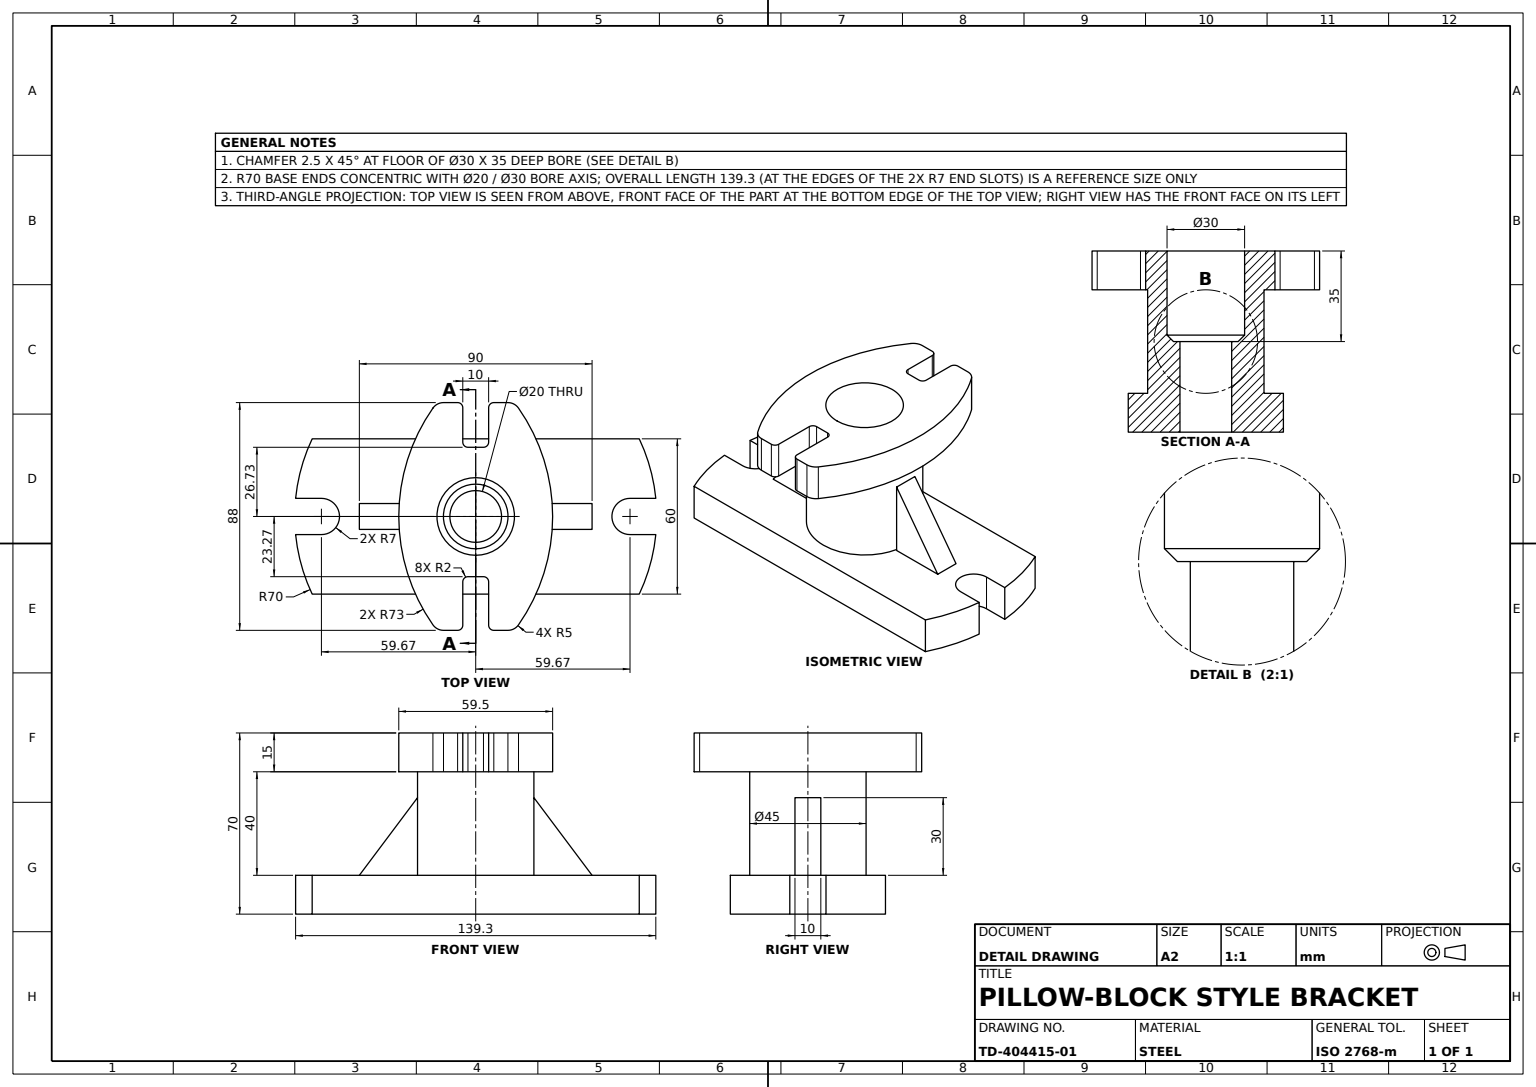
from build123d import *

# Parameters (mm, degrees)
BASE_PLATE_DEPTH         = 15
BOSS_SKETCH_45_R         = 22.5
BOSS_45_DEPTH            = 40
TOP_FLANGE_DEPTH         = 15
COUNTERBORE_SKETCH_30_R  = 15
COUNTERBORE_30_DEPTH     = 35
THROUGH_BORE_SKETCH_20_R = 10
THROUGH_BORE_20_DEPTH    = 35
BORE_CHAMFER_2_5_SIZE    = 2.5
GUSSET_RIB_DEPTH         = 5
FLANGE_FILLETS_R5_R      = 5


with BuildPart() as part:
    # Base Plate Sketch → Base Plate (new body)
    with BuildSketch(Plane(origin=(0, 0, 0), x_dir=(1, 0, 0), z_dir=(0, 1, 0))):
        with BuildLine():
            Line((-69.649120597, 7), (-59.669311209, 7))
            ThreePointArc((-59.669311209, 7), (-52.669311209, 0), (-59.669311209, -7))
            Line((-59.669311209, -7), (-69.649120597, -7))
            ThreePointArc((-69.649120597, -7), (-67.435143517, -18.775021141), (-63.245553203, -30))
            Line((-63.245553203, -30), (63.245553203, -30))
            ThreePointArc((63.245553203, -30), (67.435143517, -18.775021141), (69.649120597, -7))
            Line((69.649120597, -7), (59.669311209, -7))
            ThreePointArc((59.669311209, -7), (52.669311209, 0), (59.669311209, 7))
            Line((59.669311209, 7), (69.649120597, 7))
            ThreePointArc((69.649120597, 7), (67.435143517, 18.775021141), (63.245553203, 30))
            Line((63.245553203, 30), (-63.245553203, 30))
            ThreePointArc((-63.245553203, 30), (-67.435143517, 18.775021141), (-69.649120597, 7))
        make_face()
    extrude(amount=BASE_PLATE_DEPTH)

    # Boss Sketch Ø45 → Boss Ø45 (add)
    with BuildSketch(Plane(origin=(0, 15, 0), x_dir=(1, 0, 0), z_dir=(0, 1, 0))):
        with Locations(Location((0, 0, 0), (0, 0, 270))):
            Circle(BOSS_SKETCH_45_R)
    extrude(amount=BOSS_45_DEPTH)

    # Top Flange Sketch → Top Flange (add)
    with BuildSketch(Plane(origin=(0, 55, 0), x_dir=(1, 0, 0), z_dir=(0, 1, 0))):
        with BuildLine():
            Line((7, -44), (15, -44))
            ThreePointArc((15, -44), (29.750536483, 0), (15, 44))
            Line((15, 44), (7, 44))
            ThreePointArc((7, 44), (5.585786438, 43.414213562), (5, 42))
            Line((5, 42), (5, 25.266861381))
            ThreePointArc((5, 25.266861381), (4.414213562, 23.852647819), (3, 23.266861381))
            Line((3, 23.266861381), (-3, 23.266861381))
            ThreePointArc((-3, 23.266861381), (-4.414213562, 23.852647819), (-5, 25.266861381))
            Line((-5, 25.266861381), (-5, 42))
            ThreePointArc((-5, 42), (-5.585786438, 43.414213562), (-7, 44))
            Line((-7, 44), (-15, 44))
            ThreePointArc((-15, 44), (-29.750536483, 0), (-15, -44))
            Line((-15, -44), (-7, -44))
            ThreePointArc((-7, -44), (-5.585786438, -43.414213562), (-5, -42))
            Line((-5, -42), (-5, -28.733138619))
            ThreePointArc((-5, -28.733138619), (-4.414213562, -27.318925056), (-3, -26.733138619))
            Line((-3, -26.733138619), (3, -26.733138619))
            ThreePointArc((3, -26.733138619), (4.414213562, -27.318925056), (5, -28.733138619))
            Line((5, -28.733138619), (5, -42))
            ThreePointArc((5, -42), (5.585786438, -43.414213562), (7, -44))
        make_face()
    extrude(amount=TOP_FLANGE_DEPTH)

    # Counterbore Sketch Ø30 → Counterbore Ø30 (cut)
    with BuildSketch(Plane(origin=(0, 70, 0), x_dir=(1, 0, 0), z_dir=(0, 1, 0))):
        with Locations(Location((0, 0, 0), (0, 0, 270))):
            Circle(COUNTERBORE_SKETCH_30_R)
    extrude(amount=-COUNTERBORE_30_DEPTH, mode=Mode.SUBTRACT)

    # Through Bore Sketch Ø20 → Through Bore Ø20 (cut)
    with BuildSketch(Plane(origin=(0, 35, 0), x_dir=(1, 0, 0), z_dir=(0, 1, 0))):
        with Locations(Location((0, 0, 0), (0, 0, 270))):
            Circle(THROUGH_BORE_SKETCH_20_R)
    extrude(amount=-THROUGH_BORE_20_DEPTH, mode=Mode.SUBTRACT)

    # Bore Chamfer 2.5
    bore_chamfer_2_5_edges = [part.edges().sort_by_distance(p)[0] for p in [
        (0, 35, -15),
    ]]
    chamfer(bore_chamfer_2_5_edges, length=BORE_CHAMFER_2_5_SIZE)

    # Flange Fillets R5
    flange_fillets_r5_edges = [part.edges().sort_by_distance(p)[0] for p in [
        (15, 62.5, 44),
        (15, 62.5, -44),
        (-15, 62.5, -44),
        (-15, 62.5, 44),
    ]]
    fillet(flange_fillets_r5_edges, radius=FLANGE_FILLETS_R5_R)


with BuildPart() as body_2:
    # Gusset Rib Sketch → Gusset Rib (new, symmetric)
    with BuildSketch(Plane.XY):
        Polygon((-22.5, 45), (-22.5, 15), (-45, 15), align=None)
    extrude(amount=GUSSET_RIB_DEPTH, both=True)


with BuildPart() as body_3:
    # Gusset Rib Mirror: mirrored copy
    add(body_2.part.mirror(Plane(origin=(0, 0, 0), x_dir=(0, 0, 1), z_dir=(1, 0, 0))))


solid = Compound([part.part, body_2.part, body_3.part])
